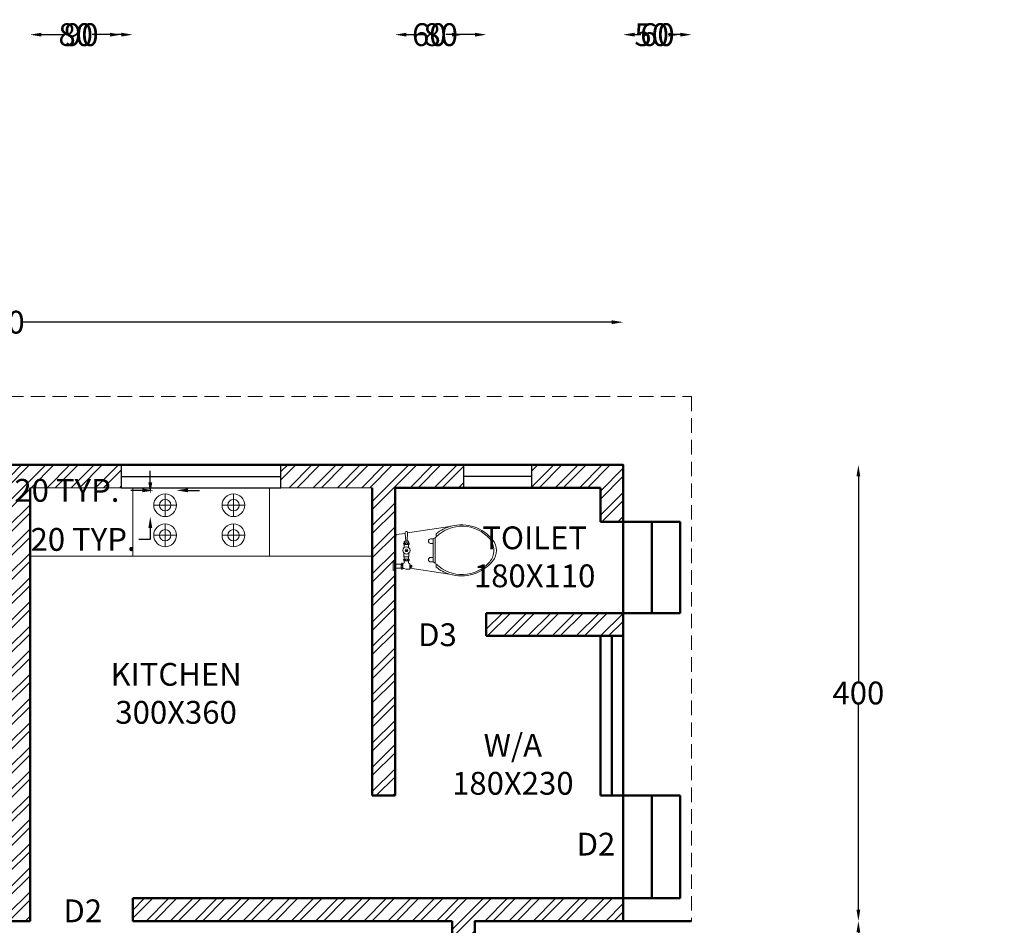
# Model space of a CAD drawing. Units: centimetres. Extents: x 10444 to 13814, y 8288 to 11191.
# Tile 6 of 9: x 11266 to 12129, y 10397 to 11191. Entities that reach past the tile are written whole.
import ezdxf

# ---------------------------------------------------------------- set-up
doc = ezdxf.new("R2010")
doc.units = ezdxf.units.CM
doc.header["$MEASUREMENT"] = 0
doc.linetypes.add('DASHED', pattern=[19.05, 12.7, -6.35])
for name, color, linetype, lineweight in [('A-ANNO-DIMS', 2, 'Continuous', 18), ('A-ANNO-TEXT', 7, 'Continuous', 25), ('A-AREA-IDEN', 3, 'Continuous', 25), ('A-FLOR-FIXT', 9, 'Continuous', 18), ('A-GLAZ', 4, 'Continuous', 25), ('A-ROOF-OVHD', 6, 'DASHED', 18), ('A-WALL', 7, 'Continuous', 50), ('A-WALL-PATT', 8, 'Continuous', 13)]:
    doc.layers.add(name, color=color, linetype=linetype, lineweight=lineweight)
doc.styles.get("Standard").update_dxf_attribs({"font": 'arial.ttf'})
doc.dimstyles.get("Standard").update_dxf_attribs({"dimtxt": 20, "dimasz": 10, "dimexe": 0.18, "dimexo": 0.0625, "dimgap": 0.09, "dimtad": 0, "dimtih": 1, "dimtoh": 1, "dimdec": 0, "dimzin": 0, "dimdsep": 46, "dimtxsty": 'Standard', "dimcen": 0.09, "dimse1": 1, "dimse2": 1, "dimadec": 0, "dimazin": 0, "dimtfac": 1, "dimtdec": 0, "dimtofl": 0, "dimtmove": 0, "dimatfit": 3, "dimfxl": 1, "dimtolj": 1, "dimtzin": 0, "dimarcsym": 0})

# ---------------------------------------------------------------- blocks, each defined once
blk = doc.blocks.new('TOILETY')
for p, q in [((2296.18, 1053.04), (2296.18, 1053.32)), ((2296.61, 1052.51), (2296.98, 1052.51)), ((2296.98, 1052.51), (2297.74, 1052.51)), ((2297.74, 1052.61), (2297.74, 1052.53)), ((2297.74, 1052.53), (2297.74, 1052.51)), ((2297.74, 1052.51), (2297.74, 1050.24)), ((2303.23, 1052.05), (2303.23, 1050.7)), ((2307.26, 1052.61), (2307.26, 1052.53)), ((2307.26, 1052.53), (2307.26, 1052.51)), ((2307.26, 1052.51), (2307.26, 1050.24)), ((2297.74, 1050.24), (2297.74, 1050.17)), ((2307.26, 1050.24), (2307.26, 1050.17)), ((2296.53, 1036.19), (2297.18, 1037.38)), ((2297.18, 1037.38), (2297.18, 1038.67)), ((2299.5, 1037.38), (2297.18, 1037.38)), ((2299.5, 1038.67), (2299.5, 1037.38)), ((2303.22, 1037.38), (2299.5, 1037.38)), ((2303.22, 1037.38), (2306.94, 1037.38)), ((2306.94, 1038.67), (2306.94, 1037.38)), ((2306.94, 1037.38), (2309.26, 1037.38)), ((2309.26, 1037.38), (2309.26, 1038.67)), ((2309.9, 1036.19), (2309.26, 1037.38))]:
    blk.add_line(p, q)
for points in [[(2293.85, 1057.29), (2293.28, 1057.29, -0.293225), (2292.64, 1058.42), (2294.98, 1058.42), (2297.17, 1058.42, -0.293225), (2296.54, 1057.29), (2295.97, 1057.29)], [(2294.98, 1057.29), (2293.85, 1057.29, -0.293225)], [(2294.98, 1057.29), (2295.97, 1057.29, 0.335115)], [(2295.97, 1056.9, -0.066772), (2311.57, 1056.74, -11.173493)], [(2312.2, 1051.98), (2311.57, 1056.74, 0.064477)], [(2293.85, 1054.1), (2293.63, 1054.1, 0.913215), (2293.63, 1053.32)], [(2294.91, 1054.1), (2293.85, 1054.1, 0.913215)], [(2294.91, 1054.1), (2295.97, 1054.1, -0.913215)], [(2295.97, 1054.1), (2296.18, 1054.1, -0.913215), (2296.18, 1053.32), (2296.11, 1053.32)], [(2297.78, 1052.66, 0.071269), (2297.81, 1052.53, 0.085783), (2297.9, 1052.35, 0.10607), (2298.04, 1052.23, 0.126822), (2298.2, 1052.19, 0.126822), (2298.36, 1052.23, 0.10607), (2298.5, 1052.35, 0.085783), (2298.59, 1052.53, 0.071269), (2298.62, 1052.66, 0.075445)], [(2298.66, 1052.58, 0.236068), (2298.84, 1052.47), (2299.76, 1052.47, 0.868488)], [(2306.34, 1052.58, -0.236068), (2306.17, 1052.47), (2304.79, 1052.47, -0.947474)], [(2307.23, 1052.66, -0.071269), (2307.19, 1052.53, -0.085783), (2307.1, 1052.35, -0.10607), (2306.96, 1052.23, -0.126822), (2306.8, 1052.19, -0.126822), (2306.65, 1052.23, -0.10607), (2306.5, 1052.35, -0.085783), (2306.41, 1052.53, -0.071269), (2306.38, 1052.66, -0.075445)], [(2307.26, 1052.51, 0.414214), (2307.4, 1052.44), (2307.9, 1052.47, -0.274044), (2308.04, 1052.4), (2308.04, 1051.9)], [(2308.04, 1051.9, 0.386607), (2308.25, 1051.76), (2312.2, 1051.98, -0.016038)], [(2312.2, 1051.98), (2312.68, 1052.01, -0.016603), (2312.71, 1052.01, -1.33807)], [(2312.71, 1052.01, -0.398884), (2313.25, 1051.55), (2313.25, 1051.37)], [(2312.71, 1050.74, 0.398884), (2313.25, 1051.2), (2313.25, 1051.37)], [(2290.73, 1028.75), (2293.96, 1049.64, -0.075157)], [(2297.78, 1050.12, -0.056795), (2297.81, 1050.29, -0.085783), (2297.9, 1050.46, -0.10607), (2298.04, 1050.59, -0.126822), (2298.2, 1050.63, -0.126822), (2298.36, 1050.59, -0.10607), (2298.5, 1050.46, -0.085783), (2298.59, 1050.29, -0.056795), (2298.62, 1050.12, -0.075445)], [(2298.66, 1050.17, -0.236068), (2298.84, 1050.28), (2299.76, 1050.28, -0.868488)], [(2306.34, 1050.17, 0.236068), (2306.17, 1050.28), (2304.79, 1050.28, 0.947474)], [(2307.23, 1050.12, 0.056795), (2307.19, 1050.29, 0.085783), (2307.1, 1050.46, 0.10607), (2306.96, 1050.59, 0.126822), (2306.8, 1050.63, 0.126822), (2306.65, 1050.59, 0.10607), (2306.5, 1050.46, 0.085783), (2306.41, 1050.29, 0.056795), (2306.38, 1050.12, 0.075445)], [(2307.26, 1050.24, -0.414214), (2307.4, 1050.31), (2307.9, 1050.28, 0.274044), (2308.04, 1050.35), (2308.04, 1050.84)], [(2308.04, 1050.84, -0.386607), (2308.25, 1050.98), (2312.4, 1050.75, 0.016063)], [(2312.4, 1050.75), (2312.68, 1050.74, 0.016603), (2312.71, 1050.74, 1.33807)], [(2315.84, 1028.5), (2312.4, 1050.75, 0.07524)], [(2296.03, 1035.7, 0.434217), (2297.18, 1007.59, 0.182634), (2303.22, 1005.38, 2.693815)], [(2294.42, 1035.7, 0.094048), (2290.73, 1028.75, 0.16845)], [(2296.03, 1035.7), (2294.42, 1035.7, 0.416606)], [(2296.53, 1036.19, 0.008985), (2296.03, 1035.7, 0.182634)], [(2303.22, 1036.19), (2296.53, 1036.19, 0.008985)], [(2303.22, 1036.19), (2309.9, 1036.19, -0.444938)], [(2310.4, 1035.7, -0.434217), (2309.26, 1007.59, -0.182634), (2303.22, 1005.38, -2.693815)], [(2309.9, 1036.19, -0.008985), (2310.4, 1035.7, -0.182634)], [(2310.4, 1035.7), (2312.01, 1035.7, -0.416606)], [(2312.01, 1035.7, -0.105447), (2315.97, 1027.83, -0.16845)], [(2290.73, 1028.75, 0.310397), (2297.82, 1005.91, 0.16845), (2303.22, 1004.04, 2.883082)], [(2315.97, 1027.83, -0.298065), (2308.61, 1005.91, -0.16845), (2303.22, 1004.04, -2.883082)], [(2315.97, 1027.83, 0.006132), (2315.84, 1028.5, 0.069947)]]:
    blk.add_lwpolyline(points, format="xyb")
for points in [[(2293.85, 1054.1), (2293.85, 1057.29)], [(2295.97, 1056.9), (2295.97, 1057.29)], [(2295.97, 1054.1), (2295.97, 1056.9)], [(2293.63, 1053.32), (2293.63, 1052.54), (2293.28, 1051.76), (2293.28, 1049.78)], [(2296.18, 1053.32), (2293.63, 1053.32)], [(2298.66, 1050.17), (2298.66, 1052.61)], [(2299.76, 1052.51), (2299.76, 1052.72), (2301.87, 1052.72)], [(2299.76, 1052.51), (2299.76, 1050.28)], [(2306.34, 1050.17), (2306.34, 1052.61)], [(2308.04, 1051.9), (2308.04, 1051.37)], [(2308.04, 1050.84), (2308.04, 1051.37)], [(2293.96, 1049.64), (2293.35, 1049.64), (2293.28, 1049.78)], [(2294.24, 1049.64), (2293.96, 1049.64)], [(2294.17, 1049.46), (2294.24, 1049.46)], [(2294.34, 1048.89), (2294.17, 1048.89), (2294.17, 1049.46)], [(2294.17, 1049.46), (2294.45, 1049.38), (2294.81, 1049.46), (2295.16, 1049.38), (2295.44, 1049.46)], [(2294.17, 1048.89), (2294.45, 1048.96), (2294.81, 1048.89), (2295.16, 1048.96), (2295.44, 1048.89)], [(2294.24, 1049.46), (2294.24, 1049.64)], [(2295.37, 1049.64), (2294.24, 1049.64)], [(2294.24, 1049.46), (2295.37, 1049.46)], [(2294.34, 1048.89), (2294.34, 1048.51), (2294.58, 1048.51)], [(2295.26, 1048.89), (2294.34, 1048.89)], [(2294.45, 1048.96), (2294.45, 1049.38)], [(2294.58, 1048.51), (2295.26, 1048.51), (2295.26, 1048.89)], [(2295.16, 1048.96), (2295.16, 1049.38)], [(2295.37, 1049.46), (2295.44, 1049.46), (2295.44, 1048.89), (2295.26, 1048.89)], [(2296.32, 1049.78), (2296.25, 1049.64), (2295.37, 1049.64)], [(2295.37, 1049.46), (2295.37, 1049.64)], [(2296.33, 1049.78), (2296.56, 1050.24)], [(2296.56, 1050.24), (2297.74, 1050.24)], [(2299.76, 1050.28), (2299.76, 1050.06), (2301.84, 1050.06)]]:
    blk.add_lwpolyline(points)
for points in [[(2294.91, 1053.32, 0.06206), (2295.16, 1053.35, 0.075298), (2295.36, 1053.43, 0.107049), (2295.5, 1053.57, 0.150029), (2295.55, 1053.71, 0.150029), (2295.5, 1053.85, 0.107049), (2295.36, 1053.99, 0.075298), (2295.16, 1054.07, 0.06206), (2294.91, 1054.1, 0.06206), (2294.65, 1054.07, 0.075298), (2294.46, 1053.99, 0.107049), (2294.31, 1053.85, 0.150029), (2294.27, 1053.71, 0.150029), (2294.31, 1053.57, 0.107049), (2294.46, 1053.43, 0.075298), (2294.65, 1053.35, 0.06206)], [(2298.63, 1051.37, -0.075445), (2298.59, 1051.15, -0.085783), (2298.5, 1050.97, -0.10607), (2298.36, 1050.85, -0.126822), (2298.2, 1050.81, -0.126822), (2298.04, 1050.85, -0.10607), (2297.9, 1050.97, -0.085783), (2297.81, 1051.15, -0.075445), (2297.78, 1051.37, -0.075445), (2297.81, 1051.6, -0.085783), (2297.9, 1051.77, -0.10607), (2298.04, 1051.9, -0.126822), (2298.2, 1051.94, -0.126822), (2298.36, 1051.9, -0.10607), (2298.5, 1051.77, -0.085783), (2298.59, 1051.6, -0.075445)], [(2306.38, 1051.37, 0.075445), (2306.41, 1051.15, 0.085783), (2306.5, 1050.97, 0.10607), (2306.65, 1050.85, 0.126822), (2306.8, 1050.81, 0.126822), (2306.96, 1050.85, 0.10607), (2307.1, 1050.97, 0.085783), (2307.19, 1051.15, 0.075445), (2307.23, 1051.37, 0.075445), (2307.19, 1051.6, 0.085783), (2307.1, 1051.77, 0.10607), (2306.96, 1051.9, 0.126822), (2306.8, 1051.94, 0.126822), (2306.65, 1051.9, 0.10607), (2306.5, 1051.77, 0.085783), (2306.41, 1051.6, 0.075445)]]:
    blk.add_lwpolyline(points, format="xyb", close=True)
blk.add_lwpolyline([(2303.23, 1052.05), (2302.65, 1051.71), (2302.65, 1051.04), (2303.23, 1050.7), (2303.81, 1051.04), (2303.81, 1051.71)], close=True)
blk.add_circle((2303.23, 1051.37), 1.91)
for centre, radius, start, end in [((2293.74, 1053.71), 0.391, 275.1944, 84.8056), ((2296.08, 1053.71), 0.391, 95.1944, 264.8056), ((2296.71, 1053.02), 0.527, 178.4608, 258.8588), ((2298.2, 1052.31), 0.551, 33.3985, 146.6015), ((2306.8, 1052.31), 0.551, 33.3985, 146.6015), ((2298.2, 1050.47), 0.551, 213.3985, 326.6015), ((2306.8, 1050.47), 0.551, 213.3985, 326.6015), ((2298.34, 1038.67), 1.16, 0, 180), ((2308.1, 1038.67), 1.16, 0, 180)]:
    blk.add_arc(centre, radius, start, end)
blk = doc.blocks.new('*D8')
at = {"layer": 'A-ANNO-DIMS', "color": 0, "lineweight": -2, "transparency": 16777216}
for p, q in [((12001.02, 10790.63), (12001.02, 10610.94)), ((12001.02, 10410.63), (12001.02, 10590.33))]:
    blk.add_line(p, q, dxfattribs=at)
at = {"layer": 'A-ANNO-DIMS', "color": 0, "transparency": 16777216}
for points in [[(11999.35, 10790.63), (12002.69, 10790.63), (12001.02, 10800.63)], [(11999.35, 10410.63), (12002.69, 10410.63), (12001.02, 10400.63)]]:
    blk.add_solid(points, dxfattribs=at)
at = {"layer": 'Defpoints', "color": 0, "transparency": 16777216}
for p in [(11794.79, 10800.63), (11794.79, 10400.63), (12001.02, 10400.63)]:
    blk.add_point(p, dxfattribs=at)
at = {"layer": 'A-ANNO-DIMS', "color": 0, "transparency": 16777216, "insert": (12001.02, 10600.63), "char_height": 20, "attachment_point": 5}
blk.add_mtext('\\A1;400', dxfattribs=at)
blk = doc.blocks.new('*D9')
at = {"layer": 'A-ANNO-DIMS', "color": 0, "lineweight": -2, "transparency": 16777216}
for p, q in [((12001.02, 10390.63), (12001.02, 10170.94)), ((12001.02, 9930.63), (12001.02, 10150.33))]:
    blk.add_line(p, q, dxfattribs=at)
at = {"layer": 'A-ANNO-DIMS', "color": 0, "transparency": 16777216}
for points in [[(11999.35, 10390.63), (12002.69, 10390.63), (12001.02, 10400.63)], [(11999.35, 9930.63), (12002.69, 9930.63), (12001.02, 9920.63)]]:
    blk.add_solid(points, dxfattribs=at)
at = {"layer": 'Defpoints', "color": 0, "transparency": 16777216}
for p in [(11664.79, 10400.63), (11664.79, 9920.63), (12001.02, 9920.63)]:
    blk.add_point(p, dxfattribs=at)
at = {"layer": 'A-ANNO-DIMS', "color": 0, "transparency": 16777216, "insert": (12001.02, 10160.63), "char_height": 20, "attachment_point": 5}
blk.add_mtext('\\A1;480', dxfattribs=at)
blk = doc.blocks.new('*D10')
at = {"layer": 'A-ANNO-DIMS', "color": 0, "lineweight": -2, "transparency": 16777216}
for p, q in [((10694.79, 10925.83), (11210.81, 10925.83)), ((11784.79, 10925.83), (11268.77, 10925.83))]:
    blk.add_line(p, q, dxfattribs=at)
at = {"layer": 'A-ANNO-DIMS', "color": 0, "transparency": 16777216}
for points in [[(10694.79, 10927.49), (10694.79, 10924.16), (10684.79, 10925.83)], [(11784.79, 10927.49), (11784.79, 10924.16), (11794.79, 10925.83)]]:
    blk.add_solid(points, dxfattribs=at)
at = {"layer": 'Defpoints', "color": 0, "transparency": 16777216}
for p in [(11794.79, 10925.83), (10684.79, 10800.63), (11794.79, 10800.63)]:
    blk.add_point(p, dxfattribs=at)
at = {"layer": 'A-ANNO-DIMS', "color": 0, "transparency": 16777216, "insert": (11239.79, 10925.83), "char_height": 20, "attachment_point": 5}
blk.add_mtext('\\A1;1110', dxfattribs=at)
blk = doc.blocks.new('*D14')
at = {"layer": 'A-ANNO-DIMS', "color": 0, "lineweight": -2, "transparency": 16777216}
for p, q in [((11674.79, 9801.88), (11708.58, 9801.88)), ((11784.79, 9801.88), (11751, 9801.88))]:
    blk.add_line(p, q, dxfattribs=at)
at = {"layer": 'A-ANNO-DIMS', "color": 0, "transparency": 16777216}
for points in [[(11674.79, 9803.55), (11674.79, 9800.21), (11664.79, 9801.88)], [(11784.79, 9803.55), (11784.79, 9800.21), (11794.79, 9801.88)]]:
    blk.add_solid(points, dxfattribs=at)
at = {"layer": 'Defpoints', "color": 0, "transparency": 16777216}
for p in [(11664.79, 10400.63), (11794.79, 10400.63), (11664.79, 9801.88)]:
    blk.add_point(p, dxfattribs=at)
at = {"layer": 'A-ANNO-DIMS', "color": 0, "transparency": 16777216, "insert": (11729.79, 9801.88), "char_height": 20, "attachment_point": 5}
blk.add_mtext('\\A1;130', dxfattribs=at)
blk = doc.blocks.new('WIN-600')
blk.add_line((60, 10), (0, 10))
blk.add_lwpolyline([(0, 0), (60, 0), (60, 20), (0, 20)], close=True)
blk = doc.blocks.new('HOB-BURNER')
blk.add_line((20, 10), (0, 10))
blk.add_circle((10, 10), 10)
blk = doc.blocks.new('*D39')
at = {"layer": 'A-ANNO-DIMS', "color": 0, "lineweight": -2, "transparency": 16777216}
for p, q in [((11373.21, 10778.33), (11363.21, 10778.33)), ((11413.21, 10778.33), (11423.21, 10778.33))]:
    blk.add_line(p, q, dxfattribs=at)
at = {"layer": 'A-ANNO-DIMS', "color": 0, "transparency": 16777216}
for points in [[(11373.21, 10780), (11373.21, 10776.66), (11383.21, 10778.33)], [(11413.21, 10780), (11413.21, 10776.66), (11403.21, 10778.33)]]:
    blk.add_solid(points, dxfattribs=at)
at = {"layer": 'Defpoints', "color": 0, "transparency": 16777216}
for p in [(11383.21, 10778.33), (11383.21, 10775.33), (11403.21, 10775.33)]:
    blk.add_point(p, dxfattribs=at)
at = {"layer": 'A-ANNO-DIMS', "color": 0, "transparency": 16777216, "insert": (11217.96, 10778.33), "char_height": 20, "attachment_point": 5}
blk.add_mtext('\\A1;HOB BURNER 20 TYP.', dxfattribs=at)
blk = doc.blocks.new('*D40')
at = {"layer": 'A-ANNO-DIMS', "color": 0, "lineweight": -2, "transparency": 16777216}
for p, q in [((11380.21, 10785.33), (11380.21, 10795.33)), ((11380.21, 10745.33), (11380.21, 10735.33)), ((11380.21, 10735.33), (11370.21, 10735.33))]:
    blk.add_line(p, q, dxfattribs=at)
at = {"layer": 'A-ANNO-DIMS', "color": 0, "transparency": 16777216}
for points in [[(11378.54, 10785.33), (11381.88, 10785.33), (11380.21, 10775.33)], [(11378.54, 10745.33), (11381.88, 10745.33), (11380.21, 10755.33)]]:
    blk.add_solid(points, dxfattribs=at)
at = {"layer": 'Defpoints', "color": 0, "transparency": 16777216}
for p in [(11383.21, 10775.33), (11380.21, 10755.33), (11383.21, 10755.33)]:
    blk.add_point(p, dxfattribs=at)
at = {"layer": 'A-ANNO-DIMS', "color": 0, "transparency": 16777216, "insert": (11321.27, 10735.33), "char_height": 20, "attachment_point": 5}
blk.add_mtext('\\A1;20 TYP.', dxfattribs=at)
blk = doc.blocks.new('*D54')
at = {"layer": 'A-ANNO-DIMS', "color": 0, "lineweight": -2, "transparency": 16777216}
for p, q in [((11284.79, 11178), (11300.39, 11178)), ((11344.79, 11178), (11329.18, 11178))]:
    blk.add_line(p, q, dxfattribs=at)
at = {"layer": 'A-ANNO-DIMS', "color": 0, "transparency": 16777216}
for points in [[(11284.79, 11179.67), (11284.79, 11176.33), (11274.79, 11178)], [(11344.79, 11179.67), (11344.79, 11176.33), (11354.79, 11178)]]:
    blk.add_solid(points, dxfattribs=at)
at = {"layer": 'Defpoints', "color": 0, "transparency": 16777216}
for p in [(11354.79, 11178), (11354.79, 10800.63), (11274.79, 10780.63)]:
    blk.add_point(p, dxfattribs=at)
at = {"layer": 'A-ANNO-DIMS', "color": 0, "transparency": 16777216, "insert": (11314.79, 11178), "char_height": 20, "attachment_point": 5}
blk.add_mtext('\\A1;80', dxfattribs=at)
blk = doc.blocks.new('*D55')
at = {"layer": 'A-ANNO-DIMS', "color": 0, "lineweight": -2, "transparency": 16777216}
for p, q in [((11604.79, 11178), (11610.35, 11178)), ((11644.79, 11178), (11639.22, 11178))]:
    blk.add_line(p, q, dxfattribs=at)
at = {"layer": 'A-ANNO-DIMS', "color": 0, "transparency": 16777216}
for points in [[(11604.79, 11179.67), (11604.79, 11176.33), (11594.79, 11178)], [(11644.79, 11179.67), (11644.79, 11176.33), (11654.79, 11178)]]:
    blk.add_solid(points, dxfattribs=at)
at = {"layer": 'Defpoints', "color": 0, "transparency": 16777216}
for p in [(11654.79, 11178), (11654.79, 10800.63), (11594.79, 10780.63)]:
    blk.add_point(p, dxfattribs=at)
at = {"layer": 'A-ANNO-DIMS', "color": 0, "transparency": 16777216, "insert": (11624.79, 11178), "char_height": 20, "attachment_point": 5}
blk.add_mtext('\\A1;60', dxfattribs=at)
blk = doc.blocks.new('*D56')
at = {"layer": 'A-ANNO-DIMS', "color": 0, "lineweight": -2, "transparency": 16777216}
for p, q in [((11804.79, 11178), (11810.35, 11178)), ((11844.79, 11178), (11839.22, 11178))]:
    blk.add_line(p, q, dxfattribs=at)
at = {"layer": 'A-ANNO-DIMS', "color": 0, "transparency": 16777216}
for points in [[(11804.79, 11179.67), (11804.79, 11176.33), (11794.79, 11178)], [(11844.79, 11179.67), (11844.79, 11176.33), (11854.79, 11178)]]:
    blk.add_solid(points, dxfattribs=at)
at = {"layer": 'Defpoints', "color": 0, "transparency": 16777216}
for p in [(11854.79, 11178), (11854.79, 10860.63), (11794.79, 10800.63)]:
    blk.add_point(p, dxfattribs=at)
at = {"layer": 'A-ANNO-DIMS', "color": 0, "transparency": 16777216, "insert": (11824.79, 11178), "char_height": 20, "attachment_point": 5}
blk.add_mtext('\\A1;60', dxfattribs=at)
blk = doc.blocks.new('*D71')
at = {"layer": 'A-ANNO-DIMS', "color": 0, "lineweight": -2, "transparency": 16777216}
for p, q in [((10466.29, 10770.63), (10466.29, 10735.94)), ((10466.29, 10680.63), (10466.29, 10715.33))]:
    blk.add_line(p, q, dxfattribs=at)
at = {"layer": 'A-ANNO-DIMS', "color": 0, "transparency": 16777216}
for points in [[(10464.62, 10770.63), (10467.95, 10770.63), (10466.29, 10780.63)], [(10464.62, 10680.63), (10467.95, 10680.63), (10466.29, 10670.63)]]:
    blk.add_solid(points, dxfattribs=at)
at = {"layer": 'Defpoints', "color": 0, "transparency": 16777216}
for p in [(11594.79, 10780.63), (10466.29, 10670.63), (11674.79, 10670.63)]:
    blk.add_point(p, dxfattribs=at)
at = {"layer": 'A-ANNO-DIMS', "color": 0, "transparency": 16777216, "insert": (10466.29, 10725.63), "char_height": 20, "attachment_point": 5}
blk.add_mtext('\\A1;110', dxfattribs=at)
blk = doc.blocks.new('*D72')
at = {"layer": 'A-ANNO-DIMS', "color": 0, "lineweight": -2, "transparency": 16777216}
for p, q in [((11284.79, 11178), (11305.41, 11178)), ((11354.79, 11178), (11334.17, 11178))]:
    blk.add_line(p, q, dxfattribs=at)
at = {"layer": 'A-ANNO-DIMS', "color": 0, "transparency": 16777216}
for points in [[(11284.79, 11179.67), (11284.79, 11176.33), (11274.79, 11178)], [(11354.79, 11179.67), (11354.79, 11176.33), (11364.79, 11178)]]:
    blk.add_solid(points, dxfattribs=at)
at = {"layer": 'Defpoints', "color": 0, "transparency": 16777216}
for p in [(11364.79, 11178), (11274.79, 10400.63), (11364.79, 10400.63)]:
    blk.add_point(p, dxfattribs=at)
at = {"layer": 'A-ANNO-DIMS', "color": 0, "transparency": 16777216, "insert": (11319.79, 11178), "char_height": 20, "attachment_point": 5}
blk.add_mtext('\\A1;90', dxfattribs=at)
blk = doc.blocks.new('*D74')
at = {"layer": 'A-ANNO-DIMS', "color": 0, "lineweight": -2, "transparency": 16777216}
for p, q in [((11604.79, 11178), (11620.39, 11178)), ((11664.79, 11178), (11649.18, 11178))]:
    blk.add_line(p, q, dxfattribs=at)
at = {"layer": 'A-ANNO-DIMS', "color": 0, "transparency": 16777216}
for points in [[(11604.79, 11179.67), (11604.79, 11176.33), (11594.79, 11178)], [(11664.79, 11179.67), (11664.79, 11176.33), (11674.79, 11178)]]:
    blk.add_solid(points, dxfattribs=at)
at = {"layer": 'Defpoints', "color": 0, "transparency": 16777216}
for p in [(11674.79, 11178), (11594.79, 10670.63), (11674.79, 10650.63)]:
    blk.add_point(p, dxfattribs=at)
at = {"layer": 'A-ANNO-DIMS', "color": 0, "transparency": 16777216, "insert": (11634.79, 11178), "char_height": 20, "attachment_point": 5}
blk.add_mtext('\\A1;80', dxfattribs=at)
blk = doc.blocks.new('*D75')
at = {"layer": 'A-ANNO-DIMS', "color": 0, "lineweight": -2, "transparency": 16777216}
for p, q in [((10466.29, 10500.63), (10466.29, 10475.94)), ((10466.29, 10430.63), (10466.29, 10455.33))]:
    blk.add_line(p, q, dxfattribs=at)
at = {"layer": 'A-ANNO-DIMS', "color": 0, "transparency": 16777216}
for points in [[(10464.62, 10500.63), (10467.95, 10500.63), (10466.29, 10510.63)], [(10464.62, 10430.63), (10467.95, 10430.63), (10466.29, 10420.63)]]:
    blk.add_solid(points, dxfattribs=at)
at = {"layer": 'Defpoints', "color": 0, "transparency": 16777216}
for p in [(10466.29, 10510.63), (11784.79, 10510.63), (11794.79, 10420.63)]:
    blk.add_point(p, dxfattribs=at)
at = {"layer": 'A-ANNO-DIMS', "color": 0, "transparency": 16777216, "insert": (10466.29, 10465.63), "char_height": 20, "attachment_point": 5}
blk.add_mtext('\\A1;90', dxfattribs=at)
blk = doc.blocks.new('*D80')
at = {"layer": 'A-ANNO-DIMS', "color": 0, "lineweight": -2, "transparency": 16777216}
for p, q in [((11804.79, 11178), (11805.41, 11178)), ((11834.79, 11178), (11834.17, 11178))]:
    blk.add_line(p, q, dxfattribs=at)
at = {"layer": 'A-ANNO-DIMS', "color": 0, "transparency": 16777216}
for points in [[(11804.79, 11179.67), (11804.79, 11176.33), (11794.79, 11178)], [(11834.79, 11179.67), (11834.79, 11176.33), (11844.79, 11178)]]:
    blk.add_solid(points, dxfattribs=at)
at = {"layer": 'Defpoints', "color": 0, "transparency": 16777216}
for p in [(11844.79, 11178), (11794.79, 10750.63), (11844.79, 10750.63)]:
    blk.add_point(p, dxfattribs=at)
at = {"layer": 'A-ANNO-DIMS', "color": 0, "transparency": 16777216, "insert": (11819.79, 11178), "char_height": 20, "attachment_point": 5}
blk.add_mtext('\\A1;50', dxfattribs=at)

msp = doc.modelspace()

# ---------------------------------------------------------------- hatches: boundary and pattern name
at = {"layer": 'A-WALL-PATT'}
h = msp.add_hatch(dxfattribs=at)
h.set_pattern_fill('ANSI32', color=256, scale=40)
h.paths.add_polyline_path([(10809.7881, 10800.6336), (10684.7881, 10800.6336), (10684.7881, 10690.6336), (10704.7881, 10690.6336), (10704.7881, 10726.41), (10704.7881, 10780.6336), (10809.7881, 10780.6336)])
h.paths.add_polyline_path([(11154.7881, 10800.6336), (10989.7881, 10800.6336), (10989.7881, 10780.6336), (11114.7881, 10780.6336), (11154.7881, 10780.6336)])
h.paths.add_polyline_path([(11354.7881, 10800.6336), (11214.7881, 10800.6336), (11214.7881, 10780.6336), (11254.7881, 10780.6336), (11254.7881, 10582.9925, -0.00499308), (11254.7881, 10581.0383), (11254.7881, 10571.0719, -0.26947312), (11256.5873, 10571.9821), (11256.5873, 10568.3227), (11256.5873, 10564.4272, -0.26947312), (11254.7881, 10565.3375), (11254.7881, 10530.6336), (11196.6819, 10530.6336), (11196.6819, 10510.6336), (11254.7881, 10510.6336), (11254.7881, 10400.6336), (11274.7881, 10400.6336), (11274.7881, 10420.6336), (11274.7881, 10780.6336), (11354.7881, 10780.6336)])
h.paths.add_polyline_path([(10704.7881, 10510.6336), (10684.7881, 10510.6336), (10684.7881, 10400.6336), (10734.7881, 10400.6336), (10734.7881, 10340.6336), (10754.7881, 10340.6336), (10754.7881, 10400.6336), (11114.7881, 10400.6336), (11114.7881, 10420.6336), (10704.7881, 10420.6336)])
h.paths.add_polyline_path([(11794.7881, 10420.6336), (11364.7881, 10420.6336), (11364.7881, 10400.6336), (11644.7881, 10400.6336), (11644.7881, 10260.6336), (11664.7881, 10260.6336), (11664.7881, 10400.6336), (11794.7881, 10400.6336)])
h.paths.add_polyline_path([(11594.7881, 10670.6336), (11594.7881, 10708.9482, -0.26828041), (11592.9938, 10708.0455), (11592.9938, 10711.9409), (11592.9938, 10715.6003, -0.26828041), (11594.7881, 10714.6976), (11594.7881, 10780.6336), (11654.7881, 10780.6336), (11654.7881, 10800.6336), (11494.7881, 10800.6336), (11494.7881, 10780.6336), (11574.7881, 10780.6336), (11574.7881, 10510.6336), (11594.7881, 10510.6336)])
h.paths.add_polyline_path([(11794.7881, 10800.6336), (11714.7881, 10800.6336), (11714.7881, 10780.6336), (11774.7881, 10780.6336), (11774.7881, 10750.6336), (11794.7881, 10750.6336)])
h.paths.add_polyline_path([(11794.7881, 10670.6336), (11674.7881, 10670.6336), (11674.7881, 10650.6336), (11794.7881, 10650.6336)])
h.paths.add_polyline_path([(11664.7881, 10080.6336), (11644.7881, 10080.6336), (11644.7881, 9940.6336), (11549.7881, 9940.6336), (11549.7881, 9920.6336), (11664.7881, 9920.6336)])
h.paths.add_polyline_path([(11369.7881, 9940.6336), (11274.7881, 9940.6336), (11274.7881, 10300.6336), (11254.7881, 10300.6336), (11254.7881, 9940.6336), (11234.7881, 9940.6336), (11234.7881, 9920.6336), (11369.7881, 9920.6336)])
h.paths.add_polyline_path([(11094.7881, 9940.6336), (11074.7881, 9940.6336), (11074.7881, 10300.6336), (11054.7881, 10300.6336), (11054.7881, 10080.6336), (11054.7881, 9920.6336), (11094.7881, 9920.6336)])
h.paths.add_polyline_path([(11134.7881, 9940.6336), (11114.7881, 9940.6336), (11114.7881, 9920.6336), (11134.7881, 9920.6336)])
h.paths.add_polyline_path([(11174.7881, 9940.6336), (11154.7881, 9940.6336), (11154.7881, 9920.6336), (11174.7881, 9920.6336)])
h.paths.add_polyline_path([(11214.7881, 9940.6336), (11196.6819, 9940.6336), (11196.6819, 9920.6336), (11214.7881, 9920.6336)])
h.paths.add_polyline_path([(10954.7881, 10100.6336), (10874.7881, 10100.6336), (10874.7881, 10080.6336), (10954.7881, 10080.6336)])
h.paths.add_polyline_path([(10814.7881, 10100.6336), (10754.7881, 10100.6336), (10754.7881, 10160.6336), (10734.7881, 10160.6336), (10734.7881, 10080.6336), (10814.7881, 10080.6336)])
h.paths.add_polyline_path([(11255.1494, 10331.8339), (11286.882, 10331.8339), (11286.882, 10373.0481), (11255.1494, 10373.0481)], flags=9)
h.paths.add_polyline_path([(11607.8445, 10630.7128), (11653.5607, 10630.7128), (11653.5607, 10671.927), (11607.8445, 10671.927)], flags=25)
h.paths.add_polyline_path([(11746.8445, 10447.0791), (11792.5607, 10447.0791), (11792.5607, 10488.2933), (11746.8445, 10488.2933)], flags=9)
h.paths.add_polyline_path([(11296.8445, 10388.5791), (11342.5607, 10388.5791), (11342.5607, 10429.7933), (11296.8445, 10429.7933)], flags=9)
h.paths.add_polyline_path([(11376.6416, 10156.0222), (11521.6757, 10156.0222), (11521.6757, 10230.6515), (11376.6416, 10230.6515)], flags=9)
h.paths.add_polyline_path([(11437.3982, 10313.4478), (11545.1881, 10313.4478), (11545.1881, 10354.662), (11437.3982, 10354.662)], flags=25)
h.paths.add_polyline_path([(11655.4027, 10682.0329), (11777.2718, 10682.0329), (11777.2718, 10756.6623), (11655.4027, 10756.6623)], flags=9)
h.paths.add_polyline_path([(11636.2626, 10500.0811), (11758.1316, 10500.0811), (11758.1316, 10574.7105), (11636.2626, 10574.7105)], flags=9)
h.paths.add_polyline_path([(11336.6251, 10562.3234), (11469.2581, 10562.3234), (11469.2581, 10636.9528), (11336.6251, 10636.9528)], flags=9)
h = msp.add_hatch(dxfattribs=at)
h.set_pattern_fill('ANSI32', color=256, scale=40)
h.paths.add_polyline_path([(12933.1062, 10800.6336), (12768.1062, 10800.6336), (12768.1062, 10780.6336), (12933.1062, 10780.6336)])
h.paths.add_polyline_path([(12588.1062, 10800.6336), (12463.1062, 10800.6336), (12463.1062, 10780.6336), (12588.1062, 10780.6336)])
h.paths.add_polyline_path([(12483.1062, 10726.41), (12483.1062, 10780.6336), (12463.1062, 10780.6336), (12463.1062, 10690.6336), (12483.1062, 10690.6336)])
h.paths.add_polyline_path([(12483.1062, 10510.6336), (12463.1062, 10510.6336), (12463.1062, 10400.6336), (12510.094, 10400.6336), (12529.0899, 10420.6336), (12483.1062, 10420.6336)])
h.paths.add_polyline_path([(12699.6814, 10420.6336), (12529.0899, 10420.6336), (12510.094, 10400.6336), (12513.1062, 10400.6336), (12513.1062, 10340.6336), (12533.1062, 10340.6336), (12533.1062, 10400.6336), (12699.64, 10400.6336)])
h.paths.add_polyline_path([(12893.1062, 10420.6336), (12699.6814, 10420.6336), (12699.64, 10400.6336), (12893.1062, 10400.6336)])
h.paths.add_polyline_path([(13129.7438, 10800.6336), (12993.1062, 10800.6336), (12993.1062, 10780.6336), (13033.1062, 10780.6336), (13033.1062, 10600.6336), (13053.1062, 10600.6336), (13053.1062, 10780.6336), (13129.7438, 10780.6336)])
h.paths.add_polyline_path([(13433.1062, 10800.6336), (13309.7438, 10800.6336), (13309.7438, 10780.6336), (13345.5201, 10780.6336), (13353.1062, 10780.6336), (13353.1062, 10600.6336), (13373.1062, 10600.6336), (13373.1062, 10780.6336), (13433.1062, 10780.6336)])
h.paths.add_polyline_path([(13573.1062, 10800.6336), (13493.1062, 10800.6336), (13493.1062, 10780.6336), (13553.1062, 10780.6336), (13553.1062, 10600.6336), (13573.1062, 10600.6336)])
h.paths.add_polyline_path([(13573.1062, 10600.6336), (13553.1062, 10600.6336), (13553.1062, 10420.6336), (13053.1062, 10420.6336), (13053.1062, 10400.6336), (13573.1062, 10400.6336)])
h.paths.add_polyline_path([(13053.1062, 10300.6336), (13033.1062, 10300.6336), (13033.1062, 9940.6336), (13013.1062, 9940.6336), (13013.1062, 9920.6336), (13053.1062, 9920.6336)])
h.paths.add_polyline_path([(12993.1062, 9940.6336), (12975, 9940.6336), (12975, 9920.6336), (12993.1062, 9920.6336)])
h.paths.add_polyline_path([(12953.1062, 9940.6336), (12933.1062, 9940.6336), (12933.1062, 9920.6336), (12953.1062, 9920.6336)])
h.paths.add_polyline_path([(12913.1062, 9940.6336), (12893.1062, 9940.6336), (12893.1062, 9920.6336), (12913.1062, 9920.6336)])
h.paths.add_polyline_path([(12873.1062, 9940.6336), (12853.1062, 9940.6336), (12853.1062, 10300.6336), (12833.1062, 10300.6336), (12833.1062, 9920.6336), (12873.1062, 9920.6336)])
h.paths.add_polyline_path([(12733.1062, 10100.6336), (12699.0201, 10100.6336), (12698.9788, 10080.6336), (12733.1062, 10080.6336)])
h.paths.add_polyline_path([(12699.0201, 10100.6336), (12653.1062, 10100.6336), (12653.1062, 10080.6336), (12698.9788, 10080.6336)])
h.paths.add_polyline_path([(12593.1062, 10100.6336), (12533.1062, 10100.6336), (12533.1062, 10160.6336), (12513.1062, 10160.6336), (12513.1062, 10080.6336), (12593.1062, 10080.6336)])
h.paths.add_polyline_path([(13053.1062, 10600.6336), (13033.1062, 10600.6336), (13033.1062, 10576.2537, -0.00499308), (13033.1062, 10574.2995), (13033.1062, 10564.3331, -0.26947312), (13034.9053, 10565.2433), (13034.9053, 10561.5839), (13034.9053, 10557.6884, -0.26947312), (13033.1062, 10558.5987), (13033.1062, 10530.6336), (12975, 10530.6336), (12975, 10510.6336), (13053.1062, 10510.6336)])
h.paths.add_polyline_path([(12975, 10530.6336), (12893.1062, 10530.6336), (12893.1062, 10600.6336), (12873.1062, 10600.6336), (12873.1062, 10510.6336), (12975, 10510.6336)])
h.paths.add_polyline_path([(12893.1062, 10700.6336), (12873.1062, 10700.6336), (12873.1062, 10600.6336), (12893.1062, 10600.6336)])
h.paths.add_polyline_path([(13373.1062, 10600.6336), (13353.1062, 10600.6336), (13353.1062, 10507.9506), (13373.1062, 10507.9506)], flags=17)
h.paths.add_polyline_path([(13553.1062, 10620.6336), (13453.1062, 10620.6336), (13453.1062, 10600.6336), (13553.1062, 10600.6336)])
h.paths.add_polyline_path([(11114.7881, 10700.6336), (11094.7881, 10700.6336), (11094.7881, 10510.6336), (11196.6819, 10510.6336), (11196.6819, 10530.6336), (11114.7881, 10530.6336)])

# ---------------------------------------------------------------- linework, layer by layer
at = {"layer": 'A-FLOR-FIXT'}
for p, q in [((11274.7881, 10780.6336), (11574.7881, 10780.6336)), ((11364.7881, 10780.6336), (11364.7881, 10720.6336)), ((11393.2099, 10755.3306), (11393.2099, 10775.3306)), ((11453.1312, 10775.3306), (11453.1312, 10755.3306)), ((11484.7881, 10780.6336), (11484.7881, 10720.6336)), ((11393.2099, 10765.3306), (11393.2099, 10755.3306)), ((11393.2099, 10728.9464), (11393.2099, 10748.9464)), ((11453.1312, 10728.9464), (11453.1312, 10748.9464)), ((11274.7881, 10720.6336), (11574.7881, 10720.6336))]:
    msp.add_line(p, q, dxfattribs=at)
for centre in [(11393.2099, 10765.3306), (11453.1312, 10765.3306), (11393.2099, 10738.9464), (11453.1312, 10738.9464)]:
    msp.add_circle(centre, 5, dxfattribs=at)
at = {"layer": 'A-GLAZ'}
msp.add_line((11354.7881, 10790.6336), (11494.7881, 10790.6336), dxfattribs=at)
msp.add_lwpolyline([(11354.7881, 10780.6336), (11494.7881, 10780.6336), (11494.7881, 10800.6336), (11354.7881, 10800.6336)], close=True, dxfattribs=at)
at = {"layer": 'A-ROOF-OVHD'}
for p, q in [((10684.7881, 10860.6336), (11854.7881, 10860.6336)), ((11854.7881, 10860.6336), (11854.7881, 10400.6336))]:
    msp.add_line(p, q, dxfattribs=at)
at = {"layer": 'A-WALL'}
for p, q in [((10684.7881, 10800.6336), (11794.7881, 10800.6336)), ((11794.7881, 10800.6336), (11794.7881, 10750.6336)), ((11274.7881, 10780.6336), (11274.7881, 10400.6336)), ((11574.7881, 10780.6336), (11574.7881, 10510.6336)), ((11594.7881, 10780.6336), (11594.7881, 10670.6336)), ((11594.7881, 10780.6336), (11774.7881, 10780.6336)), ((11774.7881, 10780.6336), (11774.7881, 10750.6336)), ((11774.7881, 10750.6336), (11844.7881, 10750.6336)), ((11794.7881, 10750.6336), (11794.7881, 10670.6336)), ((11819.7881, 10750.6336), (11819.7881, 10670.6336)), ((11844.7881, 10750.6336), (11844.7881, 10670.6336)), ((11594.7881, 10670.6336), (11594.7881, 10510.6336)), ((11674.7881, 10670.6336), (11844.7881, 10670.6336)), ((11674.7881, 10670.6336), (11674.7881, 10650.6336)), ((11794.7881, 10670.6336), (11794.7881, 10510.6336)), ((11674.7881, 10650.6336), (11794.7881, 10650.6336)), ((11774.7881, 10650.6336), (11774.7881, 10510.6336)), ((11784.7881, 10510.6336), (11784.7881, 10650.6336)), ((11574.7881, 10510.6336), (11594.7881, 10510.6336)), ((11774.7881, 10510.6336), (11844.7881, 10510.6336)), ((11794.7881, 10510.6336), (11794.7881, 10420.6336)), ((11819.7881, 10510.6336), (11819.7881, 10420.6336)), ((11844.7881, 10510.6336), (11844.7881, 10420.6336)), ((11274.7881, 10420.6336), (11274.7881, 10400.6336)), ((11364.7881, 10420.6336), (11364.7881, 10400.6336)), ((11364.7881, 10420.6336), (11844.7881, 10420.6336)), ((11794.7881, 10420.6336), (11794.7881, 10400.6336)), ((11254.7881, 10400.6336), (11274.7881, 10400.6336)), ((11364.7881, 10400.6336), (11644.7881, 10400.6336)), ((11644.7881, 10400.6336), (11644.7881, 9940.6336)), ((11664.7881, 10400.6336), (11664.7881, 9920.6336)), ((11664.7881, 10400.6336), (11854.7881, 10400.6336))]:
    msp.add_line(p, q, dxfattribs=at)
msp.add_lwpolyline([(10734.7881, 9920.6336), (11664.7881, 9920.6336), (11664.7881, 10400.6336), (11794.7881, 10400.6336), (11794.7881, 10800.6336), (10684.7881, 10800.6336), (10684.7881, 10400.6336), (10734.7881, 10400.6336), (10734.7881, 9920.6336)], dxfattribs=at)

# ---------------------------------------------------------------- block references
at = {"layer": 'A-FLOR-FIXT', "rotation": 180}
for p in [(11403.2101, 10775.331), (11463.1314, 10775.331)]:
    msp.add_blockref('HOB-BURNER', p, dxfattribs=at)
at = {"layer": 'A-FLOR-FIXT'}
for p in [(11383.2098, 10728.946), (11443.131, 10728.946)]:
    msp.add_blockref('HOB-BURNER', p, dxfattribs=at)
at = {"layer": 'A-FLOR-FIXT', "xscale": 1.667297040358401, "yscale": 1.667297040358401, "zscale": 1.667297040358401, "rotation": 90}
msp.add_blockref('TOILETY', (13357.6919, 6885.5286), dxfattribs=at)
at = {"layer": 'A-GLAZ'}
msp.add_blockref('WIN-600', (11654.788, 10780.634), dxfattribs=at)

# ---------------------------------------------------------------- texts
at = {"layer": 'A-ANNO-TEXT', "char_height": 20, "attachment_point": 1}
for s, insert in [('D3', (11615, 10661.7155)), ('D2', (11754, 10478.0819)), ('D2', (11304, 10419.5819))]:
    msp.add_mtext_dynamic_manual_height_columns(s, width=668.5, gutter_width=1, heights=[0], dxfattribs=dict(at, insert=insert))
at = {"layer": 'A-AREA-IDEN', "char_height": 20, "attachment_point": 1}
for s, width, insert in [('\\pxqc;TOILET\\P180X110', 148.64167, (11642.8691, 10746.7237)), ('\\pxqc;KITCHEN\\P300X360', 148.64167, (11328.4979, 10627.0005)), ('\\pxqc;W/A\\P180X230', 206.523248, (11594.7881, 10564.7582))]:
    msp.add_mtext_dynamic_manual_height_columns(s, width=width, gutter_width=1, heights=[0], dxfattribs=dict(at, insert=insert))

# ---------------------------------------------------------------- dimensions: what is measured, and where the dimension line sits
at = {"layer": 'A-ANNO-DIMS'}
for base, p1, p2, picture, middle in [((11354.7881, 11178), (11274.7881, 10780.6336), (11354.7881, 10800.6336), '*D54', (11314.7881, 11178)), ((11364.7881, 11178), (11274.7881, 10400.6336), (11364.7881, 10400.6336), '*D72', (11319.7881, 11178)), ((11654.7881, 11178), (11594.7881, 10780.6336), (11654.7881, 10800.6336), '*D55', (11624.7881, 11178)), ((11674.7881, 11178), (11594.7881, 10670.6336), (11674.7881, 10650.6336), '*D74', (11634.7881, 11178)), ((11854.7881, 11178), (11794.7881, 10800.6336), (11854.7881, 10860.6336), '*D56', (11824.7881, 11178)), ((11844.7881, 11178), (11794.7881, 10750.6336), (11844.7881, 10750.6336), '*D80', (11819.7881, 11178))]:
    dim = msp.add_linear_dim(base=base, p1=p1, p2=p2, dimstyle='Standard', override={"dimdec": 0, "dimlfac": 1, "dimrnd": 0, "dimzin": 0, "dimdsep": 46, "dimlunit": 2}, dxfattribs=at)
    dim.commit()
    dim.dimension.update_dxf_attribs({"geometry": picture, "text_midpoint": middle})
for p1, p2, distance, picture, middle in [((10684.7881, 10800.6336), (11794.7881, 10800.6336), 125.1941, '*D10', (11239.7881, 10925.8277)), ((11794.7881, 10800.6336), (11794.7881, 10400.6336), 206.2322, '*D8', (12001.0203, 10600.6336)), ((11664.7881, 10400.6336), (11664.7881, 9920.6336), 336.2322, '*D9', (12001.0203, 10160.6336)), ((11794.7881, 10400.6336), (11664.7881, 10400.6336), 598.7533, '*D14', (11729.7881, 9801.8804))]:
    dim = msp.add_aligned_dim(p1=p1, p2=p2, distance=distance, dimstyle='Standard', override={"dimclrd": 0, "dimclre": 0, "dimclrt": 0}, dxfattribs=at)
    dim.commit()
    dim.dimension.update_dxf_attribs({"geometry": picture, "text_midpoint": middle})
for base, p1, p2, angle, text, picture, middle in [((11383.2099, 10778.3306), (11403.2099, 10775.3306), (11383.2099, 10775.3306), 180, 'HOB BURNER <> TYP.', '*D39', (11217.9562, 10778.3306)), ((11380.2099, 10755.3306), (11383.2099, 10775.3306), (11383.2099, 10755.3306), 270, '<> TYP.', '*D40', (11321.2727, 10735.3306))]:
    dim = msp.add_linear_dim(base=base, p1=p1, p2=p2, angle=angle, text=text, dimstyle='Standard', override={"dimdec": 0, "dimrnd": 0, "dimzin": 0, "dimlunit": 2}, dxfattribs=at)
    dim.commit()
    dim.dimension.update_dxf_attribs({"geometry": picture, "text_midpoint": middle})
for base, p1, p2, picture, middle in [((10466.2881, 10670.6336), (11594.7881, 10780.6336), (11674.7881, 10670.6336), '*D71', (10466.2881, 10725.6336)), ((10466.2881, 10510.6336), (11794.7881, 10420.6336), (11784.7881, 10510.6336), '*D75', (10466.2881, 10465.6336))]:
    dim = msp.add_linear_dim(base=base, p1=p1, p2=p2, angle=90, dimstyle='Standard', override={"dimdec": 0, "dimlfac": 1, "dimrnd": 0, "dimzin": 0, "dimdsep": 46, "dimlunit": 2}, dxfattribs=at)
    dim.commit()
    dim.dimension.update_dxf_attribs({"geometry": picture, "text_midpoint": middle})

doc.saveas('drawing.dxf')
